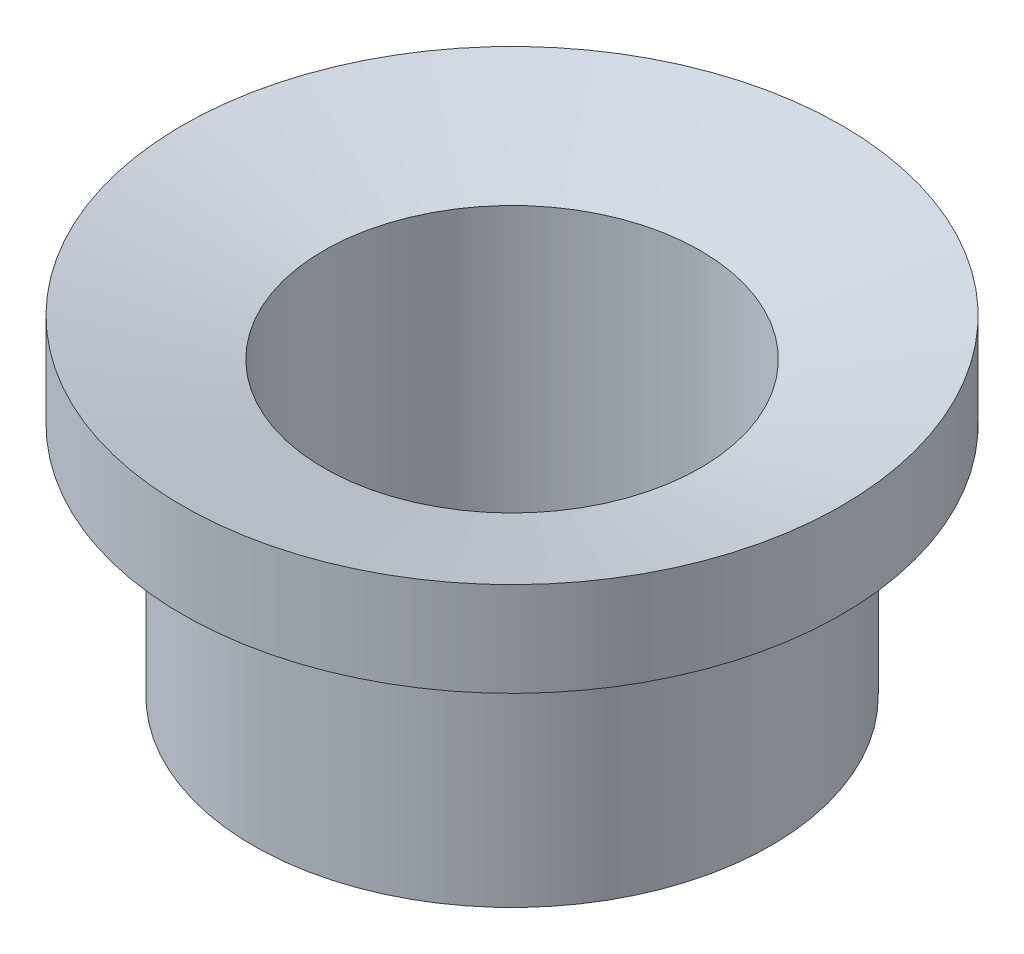
from build123d import *


with BuildPart() as part:
    # Bush Profile Sketch → Flanged Bush Revolve (revolve)
    with BuildSketch(Plane.XY, mode=Mode.PRIVATE) as flanged_bush_revolve_sk:
        Polygon((-12, 0), (-12, 18.588457268), (-21, 21), (-21, 15), (-16.5, 15), (-16.5, 0), align=None)
    revolve(flanged_bush_revolve_sk.sketch.rotate(Axis((0, -13.869565217, 0), (0, 1, 0)), 270), axis=Axis((0, -13.869565217, 0), (0, 1, 0)))


solid = part.part
